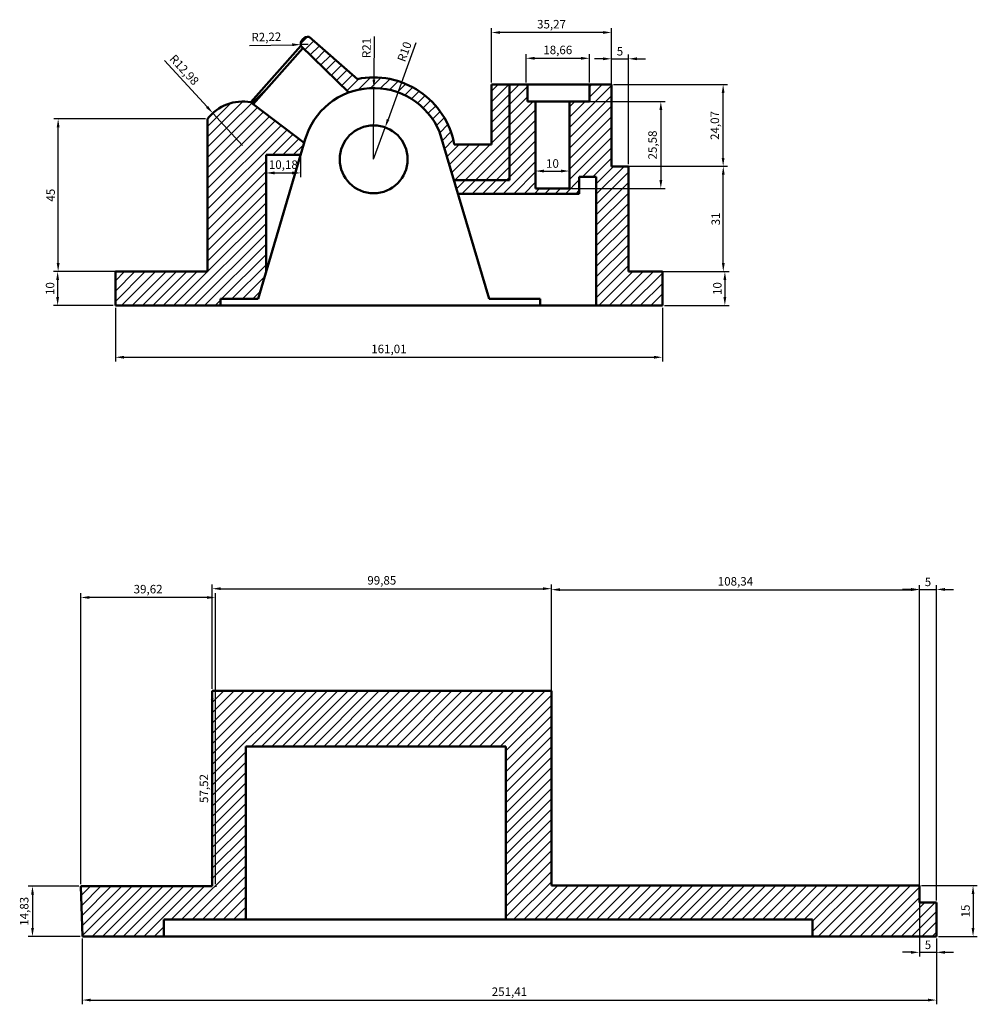
# Model space of a CAD drawing. Units: millimetres. Extents: x 1096 to 1848, y 1781 to 2075.
# Tile 2 of 2: x 1566 to 1848, y 1781 to 2071. Entities that reach past the tile are written whole.
import ezdxf

# ---------------------------------------------------------------- set-up
doc = ezdxf.new("R2010")
doc.units = ezdxf.units.MM
for name, color, linetype, lineweight in [('M-DIMS', 2, 'Continuous', 25), ('M-HATC', 8, 'Continuous', 18), ('M-OUTL', 7, 'Continuous', 50)]:
    doc.layers.add(name, color=color, linetype=linetype, lineweight=lineweight)
doc.styles.get("Standard").update_dxf_attribs({"font": 'arial.ttf'})
doc.dimstyles.new('ISO-25', dxfattribs={"dimtxt": 2.5, "dimasz": 2.5, "dimexe": 1.25, "dimexo": 0.625, "dimtad": 1, "dimtxsty": 'Standard', "dimcen": 2.5, "dimadec": 0, "dimazin": 0, "dimtfac": 1, "dimtmove": 0, "dimatfit": 3, "dimfxl": 1, "dimarcsym": 0})

# ---------------------------------------------------------------- blocks, each defined once
blk = doc.blocks.new('*D13')
at = {"layer": 'Defpoints', "color": 0, "transparency": 16777216}
for p in [(1594.4, 1987.07), (1755.42, 1987.07), (1755.42, 1971.84)]:
    blk.add_point(p, dxfattribs=at)
at = {"layer": 'M-DIMS', "color": 0, "lineweight": -2, "transparency": 16777216}
for p, q in [((1594.4, 1986.44), (1594.4, 1970.59)), ((1755.42, 1986.44), (1755.42, 1970.59)), ((1596.9, 1971.84), (1752.92, 1971.84))]:
    blk.add_line(p, q, dxfattribs=at)
at = {"layer": 'M-DIMS', "color": 0, "transparency": 16777216}
for points in [[(1596.9, 1972.26), (1596.9, 1971.43), (1594.4, 1971.84)], [(1752.92, 1972.26), (1752.92, 1971.43), (1755.42, 1971.84)]]:
    blk.add_solid(points, dxfattribs=at)
at = {"layer": 'M-DIMS', "color": 0, "transparency": 16777216, "insert": (1674.91, 1973.97), "char_height": 2.5, "attachment_point": 5}
blk.add_mtext('161,01', dxfattribs=at)
blk = doc.blocks.new('*D14')
at = {"layer": 'Defpoints', "color": 0, "transparency": 16777216}
for p in [(1755.42, 1997.07), (1755.42, 1987.07), (1773.8, 1987.07)]:
    blk.add_point(p, dxfattribs=at)
at = {"layer": 'M-DIMS', "color": 0, "lineweight": -2, "transparency": 16777216}
for p, q in [((1756.04, 1997.07), (1775.05, 1997.07)), ((1773.8, 1994.57), (1773.8, 1989.57)), ((1756.04, 1987.07), (1775.05, 1987.07))]:
    blk.add_line(p, q, dxfattribs=at)
at = {"layer": 'M-DIMS', "color": 0, "transparency": 16777216}
for points in [[(1773.38, 1994.57), (1774.21, 1994.57), (1773.8, 1997.07)], [(1773.38, 1989.57), (1774.21, 1989.57), (1773.8, 1987.07)]]:
    blk.add_solid(points, dxfattribs=at)
at = {"layer": 'M-DIMS', "color": 0, "transparency": 16777216, "insert": (1771.9, 1992.07), "char_height": 2.5, "attachment_point": 5, "rotation": 90}
blk.add_mtext('10', dxfattribs=at)
blk = doc.blocks.new('*D15')
at = {"layer": 'Defpoints', "color": 0, "transparency": 16777216}
for p in [(1745.42, 2028.07), (1773.33, 2028.07), (1745.42, 1997.07)]:
    blk.add_point(p, dxfattribs=at)
at = {"layer": 'M-DIMS', "color": 0, "lineweight": -2, "transparency": 16777216}
for p, q in [((1746.04, 2028.07), (1774.58, 2028.07)), ((1773.33, 1999.57), (1773.33, 2025.57)), ((1746.04, 1997.07), (1774.58, 1997.07))]:
    blk.add_line(p, q, dxfattribs=at)
at = {"layer": 'M-DIMS', "color": 0, "transparency": 16777216}
for points in [[(1772.92, 2025.57), (1773.75, 2025.57), (1773.33, 2028.07)], [(1772.92, 1999.57), (1773.75, 1999.57), (1773.33, 1997.07)]]:
    blk.add_solid(points, dxfattribs=at)
at = {"layer": 'M-DIMS', "color": 0, "transparency": 16777216, "insert": (1771.43, 2012.57), "char_height": 2.5, "attachment_point": 5, "rotation": 90}
blk.add_mtext('31', dxfattribs=at)
blk = doc.blocks.new('*D16')
at = {"layer": 'Defpoints', "color": 0, "transparency": 16777216}
for p in [(1740.42, 2052.14), (1773.29, 2052.14), (1740.42, 2028.07)]:
    blk.add_point(p, dxfattribs=at)
at = {"layer": 'M-DIMS', "color": 0, "lineweight": -2, "transparency": 16777216}
for p, q in [((1741.04, 2052.14), (1774.54, 2052.14)), ((1773.29, 2030.57), (1773.29, 2049.64)), ((1741.04, 2028.07), (1774.54, 2028.07))]:
    blk.add_line(p, q, dxfattribs=at)
at = {"layer": 'M-DIMS', "color": 0, "transparency": 16777216}
for points in [[(1772.87, 2049.64), (1773.7, 2049.64), (1773.29, 2052.14)], [(1772.87, 2030.57), (1773.7, 2030.57), (1773.29, 2028.07)]]:
    blk.add_solid(points, dxfattribs=at)
at = {"layer": 'M-DIMS', "color": 0, "transparency": 16777216, "insert": (1771.16, 2040.1), "char_height": 2.5, "attachment_point": 5, "rotation": 90}
blk.add_mtext('24,07', dxfattribs=at)
blk = doc.blocks.new('*D17')
at = {"layer": 'Defpoints', "color": 0, "transparency": 16777216}
for p in [(1745.42, 2059.74), (1740.42, 2028.07), (1745.42, 2028.07)]:
    blk.add_point(p, dxfattribs=at)
at = {"layer": 'M-DIMS', "color": 0, "lineweight": -2, "transparency": 16777216}
for p, q in [((1737.92, 2059.74), (1735.42, 2059.74)), ((1740.42, 2028.69), (1740.42, 2060.99)), ((1740.42, 2059.74), (1745.42, 2059.74)), ((1745.42, 2028.69), (1745.42, 2060.99)), ((1747.92, 2059.74), (1750.42, 2059.74))]:
    blk.add_line(p, q, dxfattribs=at)
at = {"layer": 'M-DIMS', "color": 0, "transparency": 16777216}
for points in [[(1737.92, 2060.16), (1737.92, 2059.32), (1740.42, 2059.74)], [(1747.92, 2060.16), (1747.92, 2059.32), (1745.42, 2059.74)]]:
    blk.add_solid(points, dxfattribs=at)
at = {"layer": 'M-DIMS', "color": 0, "transparency": 16777216, "insert": (1742.92, 2061.64), "char_height": 2.5, "attachment_point": 5}
blk.add_mtext('5', dxfattribs=at)
blk = doc.blocks.new('*D18')
at = {"layer": 'Defpoints', "color": 0, "transparency": 16777216}
for p in [(1733.94, 2059.89), (1715.28, 2052.14), (1733.94, 2052.14)]:
    blk.add_point(p, dxfattribs=at)
at = {"layer": 'M-DIMS', "color": 0, "lineweight": -2, "transparency": 16777216}
for p, q in [((1715.28, 2052.76), (1715.28, 2061.14)), ((1717.78, 2059.89), (1731.44, 2059.89)), ((1733.94, 2052.76), (1733.94, 2061.14))]:
    blk.add_line(p, q, dxfattribs=at)
at = {"layer": 'M-DIMS', "color": 0, "transparency": 16777216}
for points in [[(1717.78, 2060.31), (1717.78, 2059.47), (1715.28, 2059.89)], [(1731.44, 2060.31), (1731.44, 2059.47), (1733.94, 2059.89)]]:
    blk.add_solid(points, dxfattribs=at)
at = {"layer": 'M-DIMS', "color": 0, "transparency": 16777216, "insert": (1724.61, 2062.02), "char_height": 2.5, "attachment_point": 5}
blk.add_mtext('18,66', dxfattribs=at)
blk = doc.blocks.new('*D19')
at = {"layer": 'Defpoints', "color": 0, "transparency": 16777216}
for p in [(1705.14, 2067.49), (1705.14, 2052.14), (1740.42, 2052.14)]:
    blk.add_point(p, dxfattribs=at)
at = {"layer": 'M-DIMS', "color": 0, "lineweight": -2, "transparency": 16777216}
for p, q in [((1705.14, 2052.76), (1705.14, 2068.74)), ((1737.92, 2067.49), (1707.64, 2067.49)), ((1740.42, 2052.76), (1740.42, 2068.74))]:
    blk.add_line(p, q, dxfattribs=at)
at = {"layer": 'M-DIMS', "color": 0, "transparency": 16777216}
for points in [[(1707.64, 2067.9), (1707.64, 2067.07), (1705.14, 2067.49)], [(1737.92, 2067.9), (1737.92, 2067.07), (1740.42, 2067.49)]]:
    blk.add_solid(points, dxfattribs=at)
at = {"layer": 'M-DIMS', "color": 0, "transparency": 16777216, "insert": (1722.78, 2069.61), "char_height": 2.5, "attachment_point": 5}
blk.add_mtext('35,27', dxfattribs=at)
blk = doc.blocks.new('*D20')
at = {"layer": 'Defpoints', "color": 0, "transparency": 16777216}
for p in [(1577.55, 2042.07), (1621.55, 2042.07), (1621.55, 1997.07)]:
    blk.add_point(p, dxfattribs=at)
at = {"layer": 'M-DIMS', "color": 0, "lineweight": -2, "transparency": 16777216}
for p, q in [((1620.92, 2042.07), (1576.3, 2042.07)), ((1577.55, 1999.57), (1577.55, 2039.57)), ((1620.92, 1997.07), (1576.3, 1997.07))]:
    blk.add_line(p, q, dxfattribs=at)
at = {"layer": 'M-DIMS', "color": 0, "transparency": 16777216}
for points in [[(1577.14, 2039.57), (1577.97, 2039.57), (1577.55, 2042.07)], [(1577.14, 1999.57), (1577.97, 1999.57), (1577.55, 1997.07)]]:
    blk.add_solid(points, dxfattribs=at)
at = {"layer": 'M-DIMS', "color": 0, "transparency": 16777216, "insert": (1575.66, 2019.57), "char_height": 2.5, "attachment_point": 5, "rotation": 90}
blk.add_mtext('45', dxfattribs=at)
blk = doc.blocks.new('*D21')
at = {"layer": 'Defpoints', "color": 0, "transparency": 16777216}
for p in [(1594.4, 1997.07), (1577.4, 1987.07), (1594.4, 1987.07)]:
    blk.add_point(p, dxfattribs=at)
at = {"layer": 'M-DIMS', "color": 0, "lineweight": -2, "transparency": 16777216}
for p, q in [((1593.78, 1997.07), (1576.15, 1997.07)), ((1577.4, 1994.57), (1577.4, 1989.57)), ((1593.78, 1987.07), (1576.15, 1987.07))]:
    blk.add_line(p, q, dxfattribs=at)
at = {"layer": 'M-DIMS', "color": 0, "transparency": 16777216}
for points in [[(1576.98, 1994.57), (1577.82, 1994.57), (1577.4, 1997.07)], [(1576.98, 1989.57), (1577.82, 1989.57), (1577.4, 1987.07)]]:
    blk.add_solid(points, dxfattribs=at)
at = {"layer": 'M-DIMS', "color": 0, "transparency": 16777216, "insert": (1575.5, 1992.07), "char_height": 2.5, "attachment_point": 5, "rotation": 90}
blk.add_mtext('10', dxfattribs=at)
blk = doc.blocks.new('*D22')
at = {"layer": 'Defpoints', "color": 0, "transparency": 16777216}
for p in [(1670.49, 2051.14), (1670.42, 2030.14)]:
    blk.add_point(p, dxfattribs=at)
at = {"layer": 'M-DIMS', "color": 0, "lineweight": -2, "transparency": 16777216}
for p, q in [((1670.54, 2066.28), (1670.5, 2053.64)), ((1670.42, 2030.14), (1670.49, 2051.14))]:
    blk.add_line(p, q, dxfattribs=at)
at = {"layer": 'M-DIMS', "color": 0, "transparency": 16777216}
blk.add_solid([(1670.08, 2053.64), (1670.91, 2053.64), (1670.49, 2051.14)], dxfattribs=at)
at = {"layer": 'M-DIMS', "color": 0, "transparency": 16777216, "insert": (1668.65, 2062.91), "char_height": 2.5, "attachment_point": 5, "rotation": 89.8092}
blk.add_mtext('R21', dxfattribs=at)
blk = doc.blocks.new('*D23')
at = {"layer": 'Defpoints', "color": 0, "transparency": 16777216}
for p in [(1673.81, 2039.55), (1670.42, 2030.14)]:
    blk.add_point(p, dxfattribs=at)
at = {"layer": 'M-DIMS', "color": 0, "lineweight": -2, "transparency": 16777216}
for p, q in [((1682.8, 2064.48), (1674.66, 2041.9)), ((1670.42, 2030.14), (1673.81, 2039.55))]:
    blk.add_line(p, q, dxfattribs=at)
at = {"layer": 'M-DIMS', "color": 0, "transparency": 16777216}
blk.add_solid([(1674.27, 2042.04), (1675.05, 2041.76), (1673.81, 2039.55)], dxfattribs=at)
at = {"layer": 'M-DIMS', "color": 0, "transparency": 16777216, "insert": (1679.79, 2061.73), "char_height": 2.5, "attachment_point": 5, "rotation": 70.1654}
blk.add_mtext('R10', dxfattribs=at)
blk = doc.blocks.new('*D24')
at = {"layer": 'Defpoints', "color": 0, "transparency": 16777216}
for p in [(1648.94, 2063.92), (1651.16, 2063.97)]:
    blk.add_point(p, dxfattribs=at)
at = {"layer": 'M-DIMS', "color": 0, "lineweight": -2, "transparency": 16777216}
for p, q in [((1633.83, 2063.62), (1646.44, 2063.87)), ((1651.16, 2063.97), (1648.94, 2063.92))]:
    blk.add_line(p, q, dxfattribs=at)
at = {"layer": 'M-DIMS', "color": 0, "transparency": 16777216}
blk.add_solid([(1646.43, 2064.29), (1646.45, 2063.46), (1648.94, 2063.92)], dxfattribs=at)
at = {"layer": 'M-DIMS', "color": 0, "transparency": 16777216, "insert": (1638.84, 2065.85), "char_height": 2.5, "attachment_point": 5, "rotation": 1.157}
blk.add_mtext('R2,22', dxfattribs=at)
blk = doc.blocks.new('*D25')
at = {"layer": 'Defpoints', "color": 0, "transparency": 16777216}
for p in [(1623.07, 2043.74), (1631.85, 2034.18)]:
    blk.add_point(p, dxfattribs=at)
at = {"layer": 'M-DIMS', "color": 0, "lineweight": -2, "transparency": 16777216}
for p, q in [((1608.81, 2059.28), (1621.38, 2045.58)), ((1631.85, 2034.18), (1623.07, 2043.74))]:
    blk.add_line(p, q, dxfattribs=at)
at = {"layer": 'M-DIMS', "color": 0, "transparency": 16777216}
blk.add_solid([(1621.69, 2045.86), (1621.08, 2045.3), (1623.07, 2043.74)], dxfattribs=at)
at = {"layer": 'M-DIMS', "color": 0, "transparency": 16777216, "insert": (1614.46, 2056.27), "char_height": 2.5, "attachment_point": 5, "rotation": 312.5486}
blk.add_mtext('R12,98', dxfattribs=at)
blk = doc.blocks.new('*D26')
at = {"layer": 'Defpoints', "color": 0, "transparency": 16777216}
for p in [(1728.05, 2026.68), (1718.05, 2021.56), (1728.05, 2021.56)]:
    blk.add_point(p, dxfattribs=at)
at = {"layer": 'M-DIMS', "color": 0, "lineweight": -2, "transparency": 16777216}
for p, q in [((1718.05, 2022.18), (1718.05, 2027.93)), ((1728.05, 2022.18), (1728.05, 2027.93)), ((1720.55, 2026.68), (1725.55, 2026.68))]:
    blk.add_line(p, q, dxfattribs=at)
at = {"layer": 'M-DIMS', "color": 0, "transparency": 16777216}
for points in [[(1720.55, 2027.1), (1720.55, 2026.26), (1718.05, 2026.68)], [(1725.55, 2027.1), (1725.55, 2026.26), (1728.05, 2026.68)]]:
    blk.add_solid(points, dxfattribs=at)
at = {"layer": 'M-DIMS', "color": 0, "transparency": 16777216, "insert": (1723.05, 2028.58), "char_height": 2.5, "attachment_point": 5}
blk.add_mtext('10', dxfattribs=at)
blk = doc.blocks.new('*D27')
at = {"layer": 'Defpoints', "color": 0, "transparency": 16777216}
for p in [(1728.05, 2047.14), (1728.05, 2021.56), (1754.95, 2021.56)]:
    blk.add_point(p, dxfattribs=at)
at = {"layer": 'M-DIMS', "color": 0, "lineweight": -2, "transparency": 16777216}
for p, q in [((1728.68, 2047.14), (1756.2, 2047.14)), ((1754.95, 2044.64), (1754.95, 2024.06)), ((1728.68, 2021.56), (1756.2, 2021.56))]:
    blk.add_line(p, q, dxfattribs=at)
at = {"layer": 'M-DIMS', "color": 0, "transparency": 16777216}
for points in [[(1754.54, 2044.64), (1755.37, 2044.64), (1754.95, 2047.14)], [(1754.54, 2024.06), (1755.37, 2024.06), (1754.95, 2021.56)]]:
    blk.add_solid(points, dxfattribs=at)
at = {"layer": 'M-DIMS', "color": 0, "transparency": 16777216, "insert": (1752.83, 2034.35), "char_height": 2.5, "attachment_point": 5, "rotation": 90}
blk.add_mtext('25,58', dxfattribs=at)
blk = doc.blocks.new('*D28')
at = {"layer": 'Defpoints', "color": 0, "transparency": 16777216}
for p in [(1638.74, 2031.48), (1648.93, 2031.48), (1648.93, 2026.12)]:
    blk.add_point(p, dxfattribs=at)
at = {"layer": 'M-DIMS', "color": 0, "lineweight": -2, "transparency": 16777216}
for p, q in [((1638.74, 2030.85), (1638.74, 2024.87)), ((1648.93, 2030.85), (1648.93, 2024.87)), ((1641.24, 2026.12), (1646.43, 2026.12))]:
    blk.add_line(p, q, dxfattribs=at)
at = {"layer": 'M-DIMS', "color": 0, "transparency": 16777216}
for points in [[(1641.24, 2026.54), (1641.24, 2025.71), (1638.74, 2026.12)], [(1646.43, 2026.54), (1646.43, 2025.71), (1648.93, 2026.12)]]:
    blk.add_solid(points, dxfattribs=at)
at = {"layer": 'M-DIMS', "color": 0, "transparency": 16777216, "insert": (1643.83, 2028.25), "char_height": 2.5, "attachment_point": 5}
blk.add_mtext('10,18', dxfattribs=at)
blk = doc.blocks.new('*D35')
at = {"layer": 'Defpoints', "color": 0, "transparency": 16777216}
for p in [(1584.67, 1801.26), (1836.08, 1801.26), (1836.08, 1782.54)]:
    blk.add_point(p, dxfattribs=at)
at = {"layer": 'M-DIMS', "color": 0, "lineweight": -2, "transparency": 16777216}
for p, q in [((1584.67, 1800.64), (1584.67, 1781.29)), ((1836.08, 1800.64), (1836.08, 1781.29)), ((1587.17, 1782.54), (1833.58, 1782.54))]:
    blk.add_line(p, q, dxfattribs=at)
at = {"layer": 'M-DIMS', "color": 0, "transparency": 16777216}
for points in [[(1587.17, 1782.96), (1587.17, 1782.13), (1584.67, 1782.54)], [(1833.58, 1782.96), (1833.58, 1782.13), (1836.08, 1782.54)]]:
    blk.add_solid(points, dxfattribs=at)
at = {"layer": 'M-DIMS', "color": 0, "transparency": 16777216, "insert": (1710.38, 1784.67), "char_height": 2.5, "attachment_point": 5}
blk.add_mtext('251,41', dxfattribs=at)
blk = doc.blocks.new('*D36')
at = {"layer": 'Defpoints', "color": 0, "transparency": 16777216}
for p in [(1584.22, 1816.09), (1570, 1801.26), (1584.67, 1801.26)]:
    blk.add_point(p, dxfattribs=at)
at = {"layer": 'M-DIMS', "color": 0, "lineweight": -2, "transparency": 16777216}
for p, q in [((1583.6, 1816.09), (1568.75, 1816.09)), ((1570, 1813.59), (1570, 1803.76)), ((1584.05, 1801.26), (1568.75, 1801.26))]:
    blk.add_line(p, q, dxfattribs=at)
at = {"layer": 'M-DIMS', "color": 0, "transparency": 16777216}
for points in [[(1569.59, 1813.59), (1570.42, 1813.59), (1570, 1816.09)], [(1569.59, 1803.76), (1570.42, 1803.76), (1570, 1801.26)]]:
    blk.add_solid(points, dxfattribs=at)
at = {"layer": 'M-DIMS', "color": 0, "transparency": 16777216, "insert": (1567.88, 1808.68), "char_height": 2.5, "attachment_point": 5, "rotation": 90}
blk.add_mtext('14,83', dxfattribs=at)
blk = doc.blocks.new('*D37')
at = {"layer": 'Defpoints', "color": 0, "transparency": 16777216}
for p in [(1722.75, 1903.69), (1622.9, 1873.61), (1722.75, 1873.61)]:
    blk.add_point(p, dxfattribs=at)
at = {"layer": 'M-DIMS', "color": 0, "lineweight": -2, "transparency": 16777216}
for p, q in [((1622.9, 1874.23), (1622.9, 1904.94)), ((1625.4, 1903.69), (1720.25, 1903.69)), ((1722.75, 1874.23), (1722.75, 1904.94))]:
    blk.add_line(p, q, dxfattribs=at)
at = {"layer": 'M-DIMS', "color": 0, "transparency": 16777216}
for points in [[(1625.4, 1904.11), (1625.4, 1903.28), (1622.9, 1903.69)], [(1720.25, 1904.11), (1720.25, 1903.28), (1722.75, 1903.69)]]:
    blk.add_solid(points, dxfattribs=at)
at = {"layer": 'M-DIMS', "color": 0, "transparency": 16777216, "insert": (1672.82, 1905.82), "char_height": 2.5, "attachment_point": 5}
blk.add_mtext('99,85', dxfattribs=at)
blk = doc.blocks.new('*D38')
at = {"layer": 'Defpoints', "color": 0, "transparency": 16777216}
for p in [(1622.9, 1873.61), (1622.9, 1816.09), (1622.9, 1816.09)]:
    blk.add_point(p, dxfattribs=at)
at = {"layer": 'M-DIMS', "color": 0, "lineweight": -2, "transparency": 16777216}
for p, q in [((1623.53, 1873.61), (1624.15, 1873.61)), ((1622.9, 1871.11), (1622.9, 1818.59)), ((1623.53, 1816.09), (1624.15, 1816.09))]:
    blk.add_line(p, q, dxfattribs=at)
at = {"layer": 'M-DIMS', "color": 0, "transparency": 16777216}
for points in [[(1622.48, 1871.11), (1623.32, 1871.11), (1622.9, 1873.61)], [(1622.48, 1818.59), (1623.32, 1818.59), (1622.9, 1816.09)]]:
    blk.add_solid(points, dxfattribs=at)
at = {"layer": 'M-DIMS', "color": 0, "transparency": 16777216, "insert": (1620.77, 1844.85), "char_height": 2.5, "attachment_point": 5, "rotation": 90}
blk.add_mtext('57,52', dxfattribs=at)
blk = doc.blocks.new('*D39')
at = {"layer": 'Defpoints', "color": 0, "transparency": 16777216}
for p in [(1584.22, 1901.1), (1584.22, 1816.09), (1623.84, 1816.09)]:
    blk.add_point(p, dxfattribs=at)
at = {"layer": 'M-DIMS', "color": 0, "lineweight": -2, "transparency": 16777216}
for p, q in [((1584.22, 1816.71), (1584.22, 1902.35)), ((1623.84, 1816.71), (1623.84, 1902.35)), ((1621.34, 1901.1), (1586.72, 1901.1))]:
    blk.add_line(p, q, dxfattribs=at)
at = {"layer": 'M-DIMS', "color": 0, "transparency": 16777216}
for points in [[(1586.72, 1901.51), (1586.72, 1900.68), (1584.22, 1901.1)], [(1621.34, 1901.51), (1621.34, 1900.68), (1623.84, 1901.1)]]:
    blk.add_solid(points, dxfattribs=at)
at = {"layer": 'M-DIMS', "color": 0, "transparency": 16777216, "insert": (1604.03, 1903.23), "char_height": 2.5, "attachment_point": 5}
blk.add_mtext('39,62', dxfattribs=at)
blk = doc.blocks.new('*D40')
at = {"layer": 'Defpoints', "color": 0, "transparency": 16777216}
for p in [(1831.08, 1903.4), (1722.75, 1816.26), (1831.08, 1816.26)]:
    blk.add_point(p, dxfattribs=at)
at = {"layer": 'M-DIMS', "color": 0, "lineweight": -2, "transparency": 16777216}
for p, q in [((1722.75, 1816.89), (1722.75, 1904.65)), ((1725.25, 1903.4), (1828.58, 1903.4)), ((1831.08, 1816.89), (1831.08, 1904.65))]:
    blk.add_line(p, q, dxfattribs=at)
at = {"layer": 'M-DIMS', "color": 0, "transparency": 16777216}
for points in [[(1725.25, 1903.82), (1725.25, 1902.99), (1722.75, 1903.4)], [(1828.58, 1903.82), (1828.58, 1902.99), (1831.08, 1903.4)]]:
    blk.add_solid(points, dxfattribs=at)
at = {"layer": 'M-DIMS', "color": 0, "transparency": 16777216, "insert": (1776.91, 1905.53), "char_height": 2.5, "attachment_point": 5}
blk.add_mtext('108,34', dxfattribs=at)
blk = doc.blocks.new('*D41')
at = {"layer": 'Defpoints', "color": 0, "transparency": 16777216}
for p in [(1836.08, 1903.47), (1831.08, 1811.26), (1836.08, 1811.26)]:
    blk.add_point(p, dxfattribs=at)
at = {"layer": 'M-DIMS', "color": 0, "lineweight": -2, "transparency": 16777216}
for p, q in [((1828.58, 1903.47), (1826.08, 1903.47)), ((1831.08, 1811.89), (1831.08, 1904.72)), ((1831.08, 1903.47), (1836.08, 1903.47)), ((1836.08, 1811.89), (1836.08, 1904.72)), ((1838.58, 1903.47), (1841.08, 1903.47))]:
    blk.add_line(p, q, dxfattribs=at)
at = {"layer": 'M-DIMS', "color": 0, "transparency": 16777216}
for points in [[(1828.58, 1903.89), (1828.58, 1903.05), (1831.08, 1903.47)], [(1838.58, 1903.89), (1838.58, 1903.05), (1836.08, 1903.47)]]:
    blk.add_solid(points, dxfattribs=at)
at = {"layer": 'M-DIMS', "color": 0, "transparency": 16777216, "insert": (1833.58, 1905.37), "char_height": 2.5, "attachment_point": 5}
blk.add_mtext('5', dxfattribs=at)
blk = doc.blocks.new('*D42')
at = {"layer": 'Defpoints', "color": 0, "transparency": 16777216}
for p in [(1831.08, 1816.26), (1836.08, 1801.26), (1836.08, 1796.6)]:
    blk.add_point(p, dxfattribs=at)
at = {"layer": 'M-DIMS', "color": 0, "lineweight": -2, "transparency": 16777216}
for p, q in [((1831.08, 1815.64), (1831.08, 1795.35)), ((1836.08, 1800.64), (1836.08, 1795.35)), ((1828.58, 1796.6), (1826.08, 1796.6)), ((1831.08, 1796.6), (1836.08, 1796.6)), ((1838.58, 1796.6), (1841.08, 1796.6))]:
    blk.add_line(p, q, dxfattribs=at)
at = {"layer": 'M-DIMS', "color": 0, "transparency": 16777216}
for points in [[(1828.58, 1797.01), (1828.58, 1796.18), (1831.08, 1796.6)], [(1838.58, 1797.01), (1838.58, 1796.18), (1836.08, 1796.6)]]:
    blk.add_solid(points, dxfattribs=at)
at = {"layer": 'M-DIMS', "color": 0, "transparency": 16777216, "insert": (1833.58, 1798.49), "char_height": 2.5, "attachment_point": 5}
blk.add_mtext('5', dxfattribs=at)
blk = doc.blocks.new('*D43')
at = {"layer": 'Defpoints', "color": 0, "transparency": 16777216}
for p in [(1831.08, 1816.26), (1836.08, 1801.26), (1846.85, 1801.26)]:
    blk.add_point(p, dxfattribs=at)
at = {"layer": 'M-DIMS', "color": 0, "lineweight": -2, "transparency": 16777216}
for p, q in [((1831.71, 1816.26), (1848.1, 1816.26)), ((1846.85, 1813.76), (1846.85, 1803.76)), ((1836.71, 1801.26), (1848.1, 1801.26))]:
    blk.add_line(p, q, dxfattribs=at)
at = {"layer": 'M-DIMS', "color": 0, "transparency": 16777216}
for points in [[(1846.43, 1813.76), (1847.26, 1813.76), (1846.85, 1816.26)], [(1846.43, 1803.76), (1847.26, 1803.76), (1846.85, 1801.26)]]:
    blk.add_solid(points, dxfattribs=at)
at = {"layer": 'M-DIMS', "color": 0, "transparency": 16777216, "insert": (1844.95, 1808.76), "char_height": 2.5, "attachment_point": 5, "rotation": 90}
blk.add_mtext('15', dxfattribs=at)

msp = doc.modelspace()

# ---------------------------------------------------------------- hatches: boundary and pattern name
at = {"layer": 'M-HATC'}
h = msp.add_hatch(dxfattribs=at)
h.set_pattern_fill('ANSI31', color=256, scale=0.68)
h.paths.add_polyline_path([(1638.742, 2031.479), (1648.926, 2031.479), (1649.955, 2034.98), (1634.947, 2046.39), (1634.29, 2046.921, 0.2838472), (1621.548, 2042.069), (1621.548, 1997.069), (1594.405, 1997.069), (1594.405, 1987.069), (1625.294, 1987.069), (1625.294, 1989.002), (1636.434, 1989.002), (1638.807, 1997.069), (1638.742, 1997.069)])
h.paths.add_polyline_path([(1651.485, 2066.169, 0.519186), (1648.982, 2063.529), (1663.097, 2049.821, -0.4034277), (1689.817, 2038.182), (1694.021, 2023.992), (1710.419, 2023.992), (1710.419, 2029.855), (1710.419, 2052.138), (1705.144, 2052.138), (1705.144, 2034.491), (1694.146, 2034.491, 0.4197423), (1665.62, 2053.779)])
h.paths.add_polyline_path([(1649.618, 2062.911), (1648.982, 2063.529), (1634.29, 2046.921), (1634.947, 2046.39)])
h.paths.add_polyline_path([(1740.419, 2052.138), (1733.938, 2052.138), (1733.938, 2047.138), (1728.05, 2047.138), (1728.05, 2021.556), (1718.05, 2021.556), (1718.05, 2047.138), (1715.693, 2047.138), (1715.693, 2052.138), (1710.419, 2052.138), (1710.419, 2029.855), (1710.419, 2023.992), (1694.021, 2023.992), (1695.199, 2020.018), (1730.954, 2020.018), (1730.954, 2025.018), (1735.954, 2025.018), (1735.954, 1987.069), (1755.419, 1987.069), (1755.419, 1997.069), (1745.419, 1997.069), (1745.419, 2028.069), (1740.419, 2028.069)])
h = msp.add_hatch(dxfattribs=at)
h.set_pattern_fill('ANSI31', color=256, scale=0.68)
h.paths.add_polyline_path([(1632.771, 1857.243), (1709.347, 1857.243), (1709.347, 1806.261), (1799.638, 1806.261), (1799.638, 1801.261), (1836.084, 1801.261), (1836.084, 1811.261), (1831.084, 1811.261), (1831.084, 1816.261), (1722.746, 1816.261), (1722.746, 1873.608), (1622.901, 1873.608), (1622.901, 1816.089), (1584.222, 1816.089), (1584.672, 1801.261), (1608.683, 1801.261), (1608.683, 1806.261), (1632.771, 1806.261)])

# ---------------------------------------------------------------- linework, layer by layer
at = {"layer": 'M-OUTL'}
for p, q in [((1665.62, 2053.779), (1651.485, 2066.169)), ((1648.982, 2063.529), (1634.29, 2046.921)), ((1634.947, 2046.39), (1649.618, 2062.911)), ((1648.982, 2063.529), (1663.097, 2049.821)), ((1725.419, 2052.138), (1705.144, 2052.138)), ((1705.144, 2034.491), (1705.144, 2052.138)), ((1740.419, 2052.138), (1710.419, 2052.138)), ((1710.419, 2052.138), (1710.419, 2029.855)), ((1710.419, 2052.138), (1715.693, 2052.138)), ((1715.693, 2052.138), (1715.693, 2047.138)), ((1733.938, 2047.138), (1733.938, 2052.138)), ((1740.419, 2028.069), (1740.419, 2052.138)), ((1715.693, 2047.138), (1733.938, 2047.138)), ((1718.05, 2047.138), (1718.05, 2021.556)), ((1728.05, 2021.556), (1728.05, 2047.138)), ((1634.29, 2046.921), (1634.947, 2046.39)), ((1634.947, 2046.39), (1649.955, 2034.98)), ((1621.548, 1997.069), (1621.548, 2042.069)), ((1636.434, 1989.002), (1650.349, 2036.318)), ((1704.388, 1989.002), (1689.817, 2038.182)), ((1694.146, 2034.491), (1705.144, 2034.491)), ((1638.742, 1997.069), (1638.742, 2031.479)), ((1638.742, 2031.479), (1648.926, 2031.479)), ((1710.419, 2029.855), (1710.419, 2023.992)), ((1745.419, 2028.069), (1740.419, 2028.069)), ((1745.419, 1997.069), (1745.419, 2028.069)), ((1710.419, 2023.992), (1694.021, 2023.992)), ((1735.954, 2025.018), (1730.954, 2025.018)), ((1730.954, 2025.018), (1730.954, 2020.018)), ((1735.954, 1987.069), (1735.954, 2025.018)), ((1718.05, 2021.556), (1728.05, 2021.556)), ((1730.954, 2020.018), (1695.199, 2020.018)), ((1594.405, 1997.069), (1621.548, 1997.069)), ((1594.405, 1997.069), (1594.405, 1987.069)), ((1638.742, 1997.069), (1638.807, 1997.069)), ((1755.419, 1997.069), (1745.419, 1997.069)), ((1755.419, 1987.069), (1755.419, 1997.069)), ((1594.405, 1987.069), (1755.419, 1987.069)), ((1636.434, 1989.002), (1625.294, 1989.002)), ((1625.294, 1989.002), (1625.294, 1987.069)), ((1704.388, 1989.002), (1719.388, 1989.002)), ((1719.388, 1989.002), (1719.388, 1987.069)), ((1722.746, 1873.608), (1622.901, 1873.608)), ((1622.901, 1873.608), (1622.901, 1816.089)), ((1722.746, 1816.261), (1722.746, 1873.608)), ((1632.771, 1806.261), (1632.771, 1857.243)), ((1632.771, 1857.243), (1709.347, 1857.243)), ((1709.347, 1857.243), (1709.347, 1806.261)), ((1622.901, 1816.089), (1584.222, 1816.089)), ((1584.222, 1816.089), (1584.672, 1801.261)), ((1831.084, 1816.261), (1722.746, 1816.261)), ((1831.084, 1811.261), (1831.084, 1816.261)), ((1836.084, 1811.261), (1831.084, 1811.261)), ((1836.084, 1801.261), (1836.084, 1811.261)), ((1608.683, 1801.261), (1608.683, 1806.261)), ((1608.683, 1806.261), (1799.638, 1806.261)), ((1799.638, 1806.261), (1799.638, 1801.261)), ((1584.672, 1801.261), (1836.084, 1801.261))]:
    msp.add_line(p, q, dxfattribs=at)
msp.add_circle((1670.419, 2030.138), 10, dxfattribs=at)
for centre, radius, start, end in [((1651.162, 2063.968), 2.224, 81.64836, 191.39919), ((1670.419, 2030.138), 24.123, 10.3946, 101.47402), ((1670.419, 2030.138), 21, 22.52223, 164.34131), ((1631.848, 2034.177), 12.976, 79.15186, 142.53764)]:
    msp.add_arc(centre, radius, start, end, dxfattribs=at)

# ---------------------------------------------------------------- dimensions: what is measured, and where the dimension line sits
at = {"layer": 'M-DIMS'}
for base, p1, p2, picture, middle in [((1705.14374, 2067.4865), (1740.41873, 2052.13836), (1705.14374, 2052.13836), '*D19', (1722.78124, 2069.61389)), ((1733.938, 2059.891), (1715.281, 2052.138), (1733.938, 2052.138), '*D18', (1724.61, 2062.018)), ((1745.419, 2059.739), (1740.419, 2028.069), (1745.419, 2028.069), '*D17', (1742.919, 2061.636)), ((1648.926, 2026.122), (1638.742, 2031.479), (1648.926, 2031.479), '*D28', (1643.834, 2028.249)), ((1728.05, 2026.68), (1718.05, 2021.556), (1728.05, 2021.556), '*D26', (1723.05, 2028.581)), ((1755.419, 1971.842), (1594.405, 1987.069), (1755.419, 1987.069), '*D13', (1674.912, 1973.969)), ((1722.746, 1903.6928), (1622.9006, 1873.6078), (1722.746, 1873.6078), '*D37', (1672.8233, 1905.8202)), ((1831.084, 1903.405), (1722.746, 1816.261), (1831.084, 1816.261), '*D40', (1776.915, 1905.532)), ((1836.084, 1903.471), (1831.084, 1811.261), (1836.084, 1811.261), '*D41', (1833.584, 1905.367)), ((1584.222, 1901.098), (1623.838, 1816.089), (1584.222, 1816.089), '*D39', (1604.03, 1903.225)), ((1836.084, 1796.598), (1831.084, 1816.261), (1836.084, 1801.261), '*D42', (1833.584, 1798.494)), ((1836.084, 1782.543), (1584.672, 1801.261), (1836.084, 1801.261), '*D35', (1710.378, 1784.67))]:
    dim = msp.add_linear_dim(base=base, p1=p1, p2=p2, dimstyle='ISO-25', override={"dimclrd": 0, "dimclre": 0, "dimclrt": 0}, dxfattribs=at)
    dim.commit()
    dim.dimension.update_dxf_attribs({"geometry": picture, "text_midpoint": middle})
dim = msp.add_radius_dim(center=(1651.162, 2063.968), mpoint=(1648.938, 2063.923), dimstyle='ISO-25', override={"dimclrd": 0, "dimclre": 0, "dimclrt": 0}, dxfattribs=at)
dim.commit()
dim.dimension.update_dxf_attribs({"geometry": '*D24', "text_midpoint": (1638.842, 2065.847)})
for center, mpoint, picture, middle in [((1670.419, 2030.138), (1670.489, 2051.138), '*D22', (1670.528, 2062.907)), ((1670.419, 2030.138), (1673.812, 2039.545), '*D23', (1681.58, 2061.082)), ((1631.848, 2034.177), (1623.074, 2043.736), '*D25', (1612.894, 2054.827))]:
    dim = msp.add_radius_dim(center=center, mpoint=mpoint, dimstyle='ISO-25', override={"dimclrd": 0, "dimclre": 0, "dimclrt": 0}, dxfattribs=at)
    dim.commit()
    dim.dimension.update_dxf_attribs({"geometry": picture, "text_midpoint": middle, "dimtype": 164})
for base, p1, p2, picture, middle in [((1773.288, 2052.138), (1740.419, 2028.069), (1740.419, 2052.138), '*D16', (1771.161, 2040.104)), ((1754.954, 2021.556), (1728.05, 2047.138), (1728.05, 2021.556), '*D27', (1752.827, 2034.347)), ((1577.553, 2042.069), (1621.548, 1997.069), (1621.548, 2042.069), '*D20', (1575.656, 2019.569)), ((1773.334, 2028.069), (1745.419, 1997.069), (1745.419, 2028.069), '*D15', (1771.431, 2012.569)), ((1577.401, 1987.069), (1594.405, 1997.069), (1594.405, 1987.069), '*D21', (1575.499, 1992.069)), ((1773.797, 1987.069), (1755.419, 1997.069), (1755.419, 1987.069), '*D14', (1771.896, 1992.069)), ((1622.901, 1816.089), (1622.901, 1873.608), (1622.901, 1816.089), '*D38', (1620.773, 1844.849)), ((1570.004, 1801.261), (1584.222, 1816.089), (1584.672, 1801.261), '*D36', (1567.877, 1808.675)), ((1846.848, 1801.261), (1831.084, 1816.261), (1836.084, 1801.261), '*D43', (1844.946, 1808.761))]:
    dim = msp.add_linear_dim(base=base, p1=p1, p2=p2, angle=90, dimstyle='ISO-25', override={"dimclrd": 0, "dimclre": 0, "dimclrt": 0}, dxfattribs=at)
    dim.commit()
    dim.dimension.update_dxf_attribs({"geometry": picture, "text_midpoint": middle})

doc.saveas('drawing.dxf')
